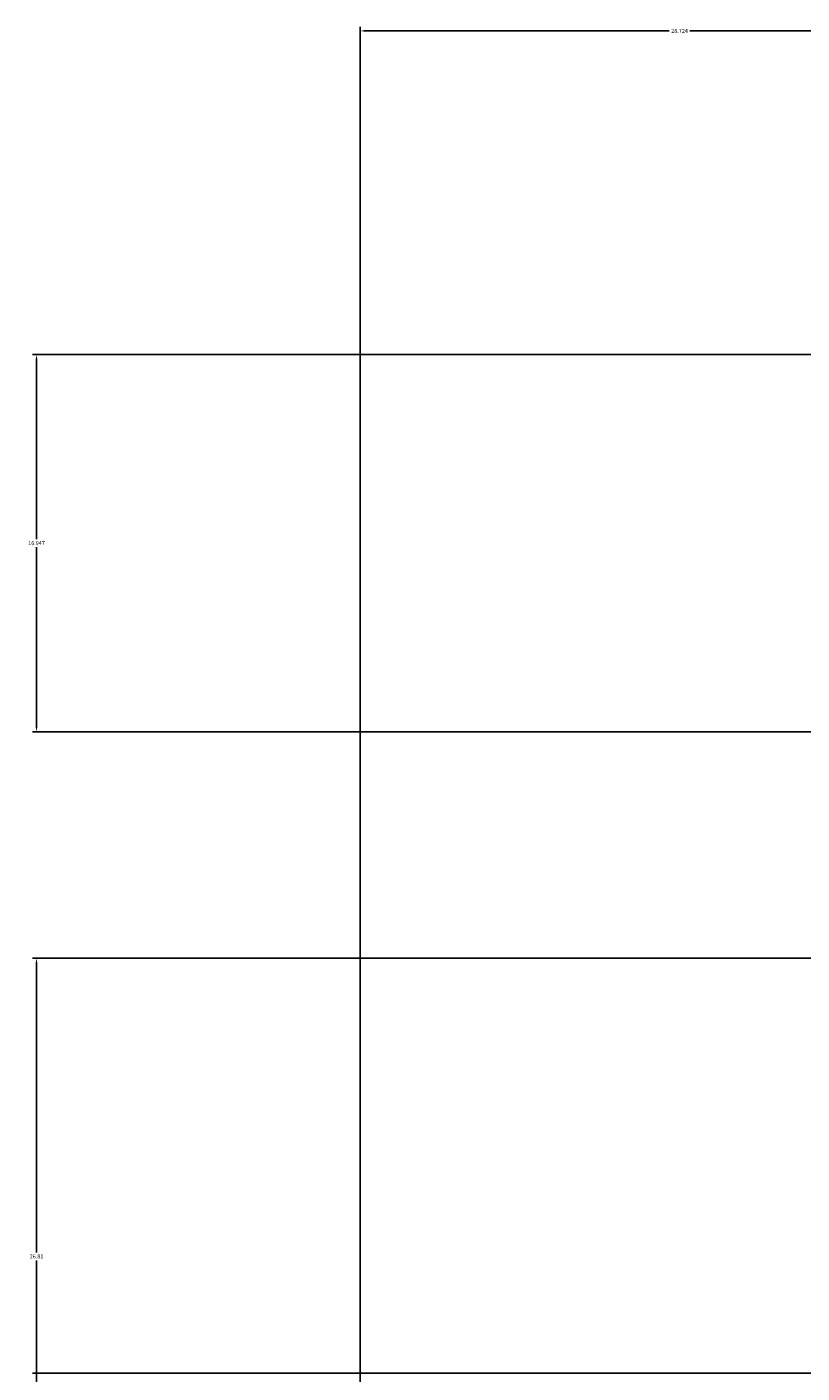
# Model space of a CAD drawing. Units: inches. Extents: x -12 to 334, y -10 to 186.
# Tile 20 of 77: x -12 to 23, y 109 to 170. Entities that reach past the tile are written whole.
import ezdxf

# ---------------------------------------------------------------- set-up
doc = ezdxf.new("R2010")
doc.units = ezdxf.units.IN
doc.header["$MEASUREMENT"] = 0
doc.layers.add('M-DIMS', color=2, linetype='Continuous', lineweight=18)
doc.styles.get("Standard").update_dxf_attribs({"font": 'arial.ttf'})
doc.dimstyles.get("Standard").update_dxf_attribs({"dimtxt": 0.18, "dimasz": 0.18, "dimexe": 0.18, "dimexo": 0.0625, "dimgap": 0.09, "dimtad": 0, "dimtih": 1, "dimtoh": 1, "dimdec": 4, "dimzin": 0, "dimdsep": 46, "dimtxsty": 'Standard', "dimcen": 0.09, "dimadec": 0, "dimazin": 0, "dimtfac": 1, "dimtdec": 4, "dimtofl": 0, "dimtmove": 0, "dimatfit": 3, "dimfxl": 1, "dimtolj": 1, "dimtzin": 0, "dimarcsym": 0})

# ---------------------------------------------------------------- blocks, each defined once
blk = doc.blocks.new('*D2')
at = {"layer": 'Defpoints', "color": 0, "transparency": 16777216}
for p in [(32.1, 169.385), (32.1, 127.708), (3.376, 80.692)]:
    blk.add_point(p, dxfattribs=at)
at = {"layer": 'M-DIMS', "color": 0, "lineweight": -2, "transparency": 16777216}
for p, q in [((3.376, 80.754), (3.376, 169.565)), ((32.1, 127.77), (32.1, 169.565)), ((3.556, 169.385), (17.274, 169.385)), ((31.92, 169.385), (18.203, 169.385))]:
    blk.add_line(p, q, dxfattribs=at)
at = {"layer": 'M-DIMS', "color": 0, "transparency": 16777216}
for points in [[(3.556, 169.415), (3.556, 169.355), (3.376, 169.385)], [(31.92, 169.415), (31.92, 169.355), (32.1, 169.385)]]:
    blk.add_solid(points, dxfattribs=at)
at = {"layer": 'M-DIMS', "color": 0, "transparency": 16777216, "insert": (17.738, 169.385), "char_height": 0.18, "attachment_point": 5}
blk.add_mtext('\\A1;28.724', dxfattribs=at)
blk = doc.blocks.new('*D8')
at = {"layer": 'Defpoints', "color": 0, "transparency": 16777216}
for p in [(-11.174, 127.708), (32.1, 127.708), (23.581, 100.896)]:
    blk.add_point(p, dxfattribs=at)
at = {"layer": 'M-DIMS', "color": 0, "lineweight": -2, "transparency": 16777216}
for p, q in [((32.038, 127.708), (-11.354, 127.708)), ((-11.174, 127.528), (-11.174, 114.484)), ((-11.174, 101.076), (-11.174, 114.12)), ((23.518, 100.896), (-11.354, 100.896))]:
    blk.add_line(p, q, dxfattribs=at)
at = {"layer": 'M-DIMS', "color": 0, "transparency": 16777216}
for points in [[(-11.204, 127.528), (-11.144, 127.528), (-11.174, 127.708)], [(-11.204, 101.076), (-11.144, 101.076), (-11.174, 100.896)]]:
    blk.add_solid(points, dxfattribs=at)
at = {"layer": 'M-DIMS', "color": 0, "transparency": 16777216, "insert": (-11.174, 114.302), "char_height": 0.18, "attachment_point": 5}
blk.add_mtext('\\A1;26.81', dxfattribs=at)
blk = doc.blocks.new('*D14')
at = {"layer": 'Defpoints', "color": 0, "transparency": 16777216}
for p in [(63.5, 109.058), (-11.174, 49.45), (64.207, 49.45)]:
    blk.add_point(p, dxfattribs=at)
at = {"layer": 'M-DIMS', "color": 0, "lineweight": -2, "transparency": 16777216}
for p, q in [((63.438, 109.058), (-11.354, 109.058)), ((-11.174, 108.878), (-11.174, 79.436)), ((-11.174, 49.63), (-11.174, 79.072)), ((64.144, 49.45), (-11.354, 49.45))]:
    blk.add_line(p, q, dxfattribs=at)
at = {"layer": 'M-DIMS', "color": 0, "transparency": 16777216}
for points in [[(-11.204, 108.878), (-11.144, 108.878), (-11.174, 109.058)], [(-11.204, 49.63), (-11.144, 49.63), (-11.174, 49.45)]]:
    blk.add_solid(points, dxfattribs=at)
at = {"layer": 'M-DIMS', "color": 0, "transparency": 16777216, "insert": (-11.174, 79.254), "char_height": 0.18, "attachment_point": 5}
blk.add_mtext('\\A1;59.61', dxfattribs=at)
blk = doc.blocks.new('*D22')
at = {"layer": 'Defpoints', "color": 0, "transparency": 16777216}
for p in [(190.342, 154.835), (-11.174, 137.887), (195.342, 137.887)]:
    blk.add_point(p, dxfattribs=at)
at = {"layer": 'M-DIMS', "color": 0, "lineweight": -2, "transparency": 16777216}
for p, q in [((190.28, 154.835), (-11.354, 154.835)), ((-11.174, 154.655), (-11.174, 146.543)), ((-11.174, 138.067), (-11.174, 146.179)), ((195.28, 137.887), (-11.354, 137.887))]:
    blk.add_line(p, q, dxfattribs=at)
at = {"layer": 'M-DIMS', "color": 0, "transparency": 16777216}
for points in [[(-11.204, 154.655), (-11.144, 154.655), (-11.174, 154.835)], [(-11.204, 138.067), (-11.144, 138.067), (-11.174, 137.887)]]:
    blk.add_solid(points, dxfattribs=at)
at = {"layer": 'M-DIMS', "color": 0, "transparency": 16777216, "insert": (-11.174, 146.361), "char_height": 0.18, "attachment_point": 5}
blk.add_mtext('\\A1;16.947', dxfattribs=at)

msp = doc.modelspace()

# ---------------------------------------------------------------- dimensions: what is measured, and where the dimension line sits
at = {"layer": 'M-DIMS'}
dim = msp.add_linear_dim(base=(32.1002, 169.3845), p1=(3.3765, 80.6915), p2=(32.1002, 127.7078), dimstyle='Standard', override={"dimdec": 3, "dimlfac": 1, "dimrnd": 0, "dimzin": 0, "dimdsep": 46, "dimlunit": 2}, dxfattribs=at)
dim.commit()
dim.dimension.update_dxf_attribs({"geometry": '*D2', "text_midpoint": (17.7383, 169.3845)})
for base, p1, p2, override, picture, middle in [((-11.1736, 137.8871), (190.3421, 154.8345), (195.3421, 137.8871), {"dimdec": 3, "dimlfac": 1, "dimrnd": 0, "dimzin": 0, "dimdsep": 46, "dimlunit": 2}, '*D22', (-11.1735, 146.3608)), ((-11.1736, 127.7078), (23.5807, 100.8958), (32.1002, 127.7078), {"dimdec": 2, "dimlfac": 1, "dimrnd": 0, "dimzin": 0, "dimdsep": 46, "dimlunit": 2}, '*D8', (-11.1735, 114.3018)), ((-11.1736, 49.4497), (63.5, 109.0583), (64.2068, 49.4497), {"dimdec": 2, "dimlfac": 1, "dimrnd": 0, "dimzin": 0, "dimdsep": 46, "dimlunit": 2}, '*D14', (-11.1735, 79.254))]:
    dim = msp.add_linear_dim(base=base, p1=p1, p2=p2, angle=90, dimstyle='Standard', override=override, dxfattribs=at)
    dim.commit()
    dim.dimension.update_dxf_attribs({"geometry": picture, "text_midpoint": middle})

doc.saveas('drawing.dxf')
